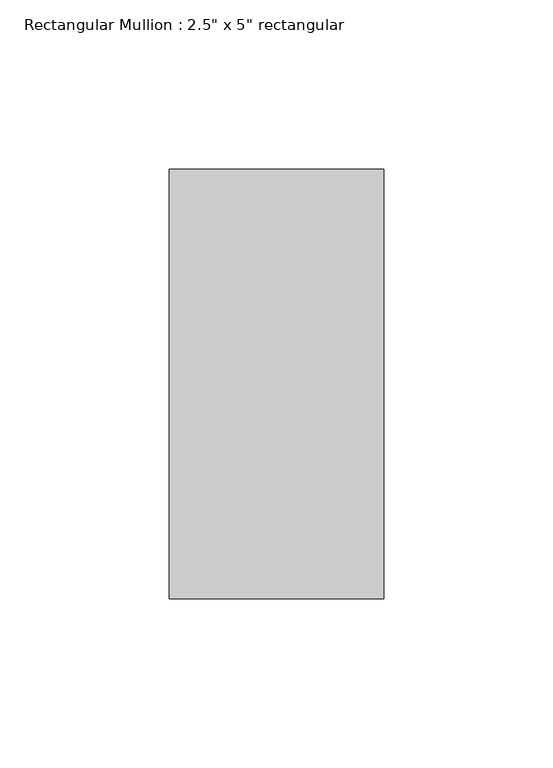
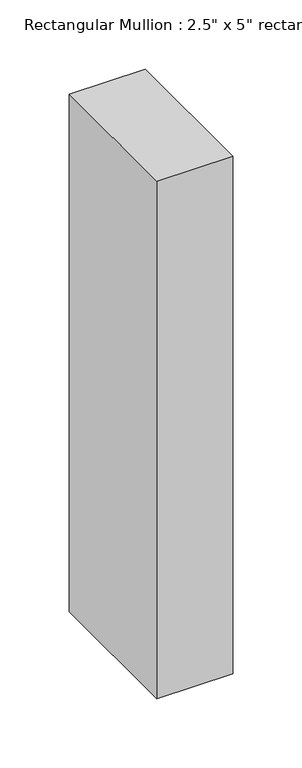
"""IFC4 building model written with IfcOpenShell, lengths in millimetres: member geometry."""

from ifc_helpers import new_model, si_unit, frame, origin, place, context, project, spatial, polyline, outline, extrude, source, transform, mapped, element, save


def member_15823cb3(model_context):
    return source(origin(), model_context, "Body", "SweptSolid", [
        extrude(outline(polyline([(0.0, 63.5), (0.0, -63.5), (-63.5, -63.5), (-63.5, 63.5), (0.0, 63.5)])), frame((0.0, 0.0, -457.2), z_axis=(0.0, 0.0, 1.0), x_axis=(1.0, 0.0, 0.0)), (0.0, 0.0, 1.0), 457.2),
    ])


if __name__ == "__main__":
    model = new_model("IFC4")
    model_context = context("Model", 3, world=origin())
    ifc_project = project(units=[si_unit("LENGTHUNIT", "METRE", prefix="MILLI")], contexts=[model_context])
    site = spatial("IfcSite", under=ifc_project)
    building = spatial("IfcBuilding", under=site)
    placement = place(None, origin())
    member_shape = member_15823cb3(model_context)
    element("IfcMember", 1, ObjectType="Rectangular Mullion : 2.5\" x 5\" rectangular", at=placement, inside=building, context=model_context, shape_type="MappedRepresentation", body=[
        mapped(member_shape, transform((0.0, 0.0, 0.0), x_axis=(1.0, 0.0, 0.0), y_axis=(0.0, 1.0, 0.0), z_axis=(0.0, 0.0, 1.0))),
    ])
    save(model, "model.ifc")

# Revit data of these elements
# Type "Rectangular Mullion : 2.5\" x 5\" rectangular"
#   built-in parameter 1007304 = 0.416667 (stored number, unit not read)
#   built-in parameter 1007301 = 0.104167 (stored number, unit not read)
#   built-in parameter 1007300 = 0.104167 (stored number, unit not read)
# Element 1 (IfcMember, "Rectangular Mullion : 2.5\" x 5\" rectangular")
#   Materials on its faces: "Aluminum"
# Materials
#   "Aluminum": class "Metal", colour RGB 247 247 247, transparency 0, Description = "Aluminum 6061", Cost = 0
